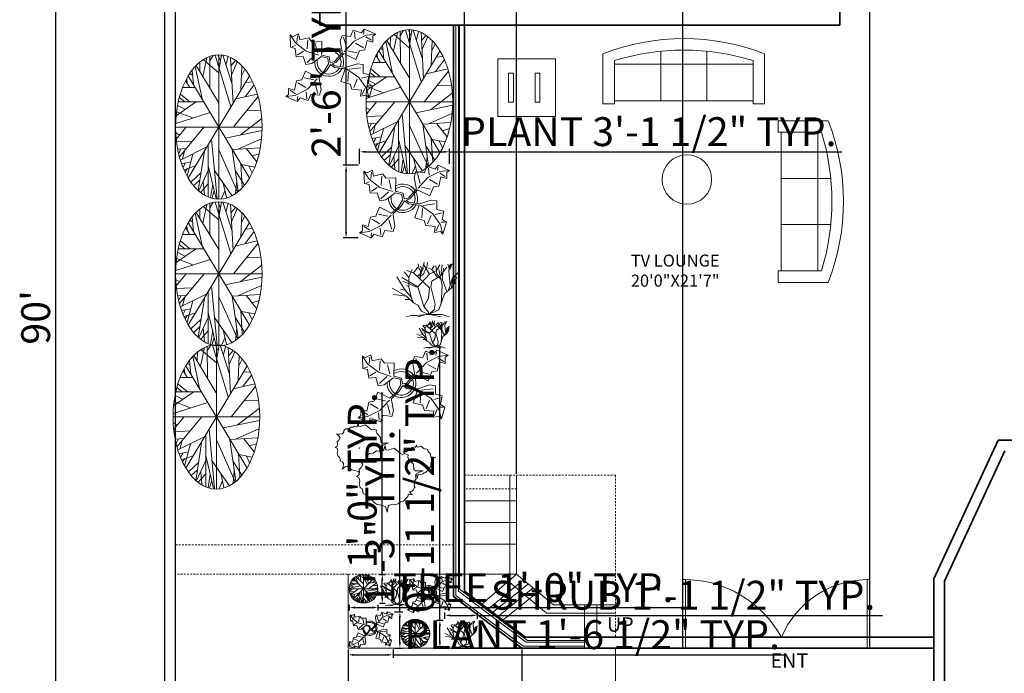
# Model space of a CAD drawing. Units: inches. Extents: x 2562 to 3392, y 1021 to 2243.
# Tile 2 of 6: x 2577 to 2986, y 1472 to 1744. Entities that reach past the tile are written whole.
import ezdxf

# ---------------------------------------------------------------- set-up
doc = ezdxf.new("R2010")
doc.units = ezdxf.units.IN
doc.linetypes.add('JIS_02_0.7', pattern=[1.35, 0.75, -0.6])
for name, color, linetype, lineweight in [('A-ANNO-DIMS', 2, 'Continuous', 18), ('A-ANNO-TEXT', 7, 'Continuous', 18), ('A-AREA-IDEN', 7, 'Continuous', 18), ('A-DOOR', 4, 'Continuous', 18), ('A-FLOR-STRS', 7, 'Continuous', 18), ('A-FLOR-STRS-HIDN', 8, 'JIS_02_0.7', 13), ('A-FURN', 8, 'Continuous', 18), ('A-GLAZ', 4, 'Continuous', 13), ('A-WALL', 7, 'Continuous', 35), ('C-PROP', 7, 'Continuous', 30), ('L-HRDS', 8, 'Continuous', 18), ('L-HRDS-HIDN', 8, 'JIS_02_0.7', 13), ('L-PLNT', 94, 'Continuous', 13)]:
    doc.layers.add(name, color=color, linetype=linetype, lineweight=lineweight)
doc.styles.get("Standard").update_dxf_attribs({"font": 'arial.ttf'})
doc.dimstyles.new('ISO-25', dxfattribs={"dimtxt": 12, "dimasz": 2.5, "dimexe": 1.25, "dimexo": 0.625, "dimtad": 1, "dimdec": 1, "dimlunit": 3, "dimtxsty": 'Standard', "dimcen": 2.5, "dimadec": 0, "dimazin": 0, "dimtfac": 1, "dimtdec": 1, "dimtmove": 0, "dimatfit": 3, "dimfxl": 1, "dimarcsym": 0})

# ---------------------------------------------------------------- blocks, each defined once
blk = doc.blocks.new('Sofa - Roundback 7 ft.')
for p, q in [((-12.00002, -32.4421), (-12.00003, -6.5971)), ((11.99997, -32.4421), (11.99998, -6.5971)), ((-36.000027, -34), (-36.000027, -11.4696)), ((-35.999844, -13.3819), (35.9998, -13.3819)), ((35.99998, -34), (35.99998, -11.4696)), ((-36.000027, -32.4421), (35.99998, -32.4421))]:
    blk.add_line(p, q)
for points in [[(-36.000027, -34), (-42.000027, -34), (-42.000027, -8)], [(41.99998, -8), (41.99998, -34), (35.99998, -34)]]:
    blk.add_lwpolyline(points)
for centre, radius, start, end in [((0, -114.25), 114.25, 68.43141, 111.5686), ((-0.00001, -127.1968), 121.1968, 72.72033, 107.2797)]:
    blk.add_arc(centre, radius, start, end)
blk = doc.blocks.new('Tree - deciduous plan')
for p, q in [((-22.0458, 42.0753), (-16.5881, 57.6486)), ((-12.5388, 54.9406), (-7.9613, 59.4546)), ((-12.3627, 32.1443), (-12.5388, 58.7776)), ((-5.3205, 59.6806), (16.5105, 16.7963)), ((2.426, 54.9406), (-1.4472, 59.9056)), ((0, 59.9996), (0, -60)), ((0.4894, 48.6208), (3.6584, 59.6806)), ((18.2711, 35.5298), (5.419, 59.6806)), ((9.8203, 51.5549), (12.8133, 58.5516)), ((19.6795, 19.5047), (16.3344, 57.6486)), ((-32.6092, 50.4264), (-23.2782, 23.5674)), ((-31.2008, 51.1035), (-0.2149, 20.1818)), ((-26.4472, 46.5894), (-26.2712, 53.8116)), ((-21.1656, 55.8436), (-0.0388, 45.0094)), ((17.0387, 51.1035), (23.2006, 55.1666)), ((17.7429, 43.6552), (25.4894, 54.2636)), ((31.6513, 50.8778), (30.2429, 30.5643)), ((42, 42), (-42, -42)), ((42, -42), (-42, 42)), ((-40.1797, 44.558), (-36.4825, 43.2038)), ((-37.0107, 47.0408), (-35.25, 35.5298)), ((31.1232, 42.5267), (35.8767, 48.1693)), ((-49.8627, 32.8214), (-32.7853, 32.8214)), ((-45.8134, 38.2383), (-40.5318, 33.0471)), ((-43.8768, 36.4326), (-44.405, 40.2696)), ((36.2288, 25.1474), (48.9049, 35.0784)), ((37.1091, 37.1098), (46.6161, 37.5612)), ((-53.2078, 27.4044), (-40.1797, 20.859)), ((54.3626, 25.3731), (20.9119, 0.3198)), ((23.3767, 23.3417), (53.3063, 27.4044)), ((-32.2571, 20.6333), (-59.1937, 9.348)), ((-57.081, 17.9248), (-47.0458, 14.7649)), ((-56.0247, 20.859), (-20.8134, 20.859)), ((-54.7923, 24.4702), (-47.75, 21.0847)), ((-59.7219, 2.8025), (-12.0106, 12.0565)), ((-58.6656, 12.7336), (-35.9543, 7.5424)), ((38.5175, 13.4107), (58.2359, 13.6364)), ((-54.6162, -24.7335), (-20.2853, 0.0941)), ((29.3626, -6.6771), (59.4682, 7.091)), ((-60, 0), (60, 0)), ((-59.7219, -4.8714), (-54.2641, -6.6771)), ((-45.2853, -0.1316), (-59.0177, -10.0627)), ((9.2922, -9.1598), (59.6443, -2.8401)), ((-58.4895, -12.3197), (-36.4825, -11.6426)), ((-14.8275, -15.0282), (-14.6515, -57.6865)), ((-10.074, -10.0627), (-2.5036, -59.7178)), ((26.3697, -18.4138), (58.9401, -9.8369)), ((-57.081, -18.4138), (-45.2853, -17.9624)), ((-52.6797, -18.188), (-55.4966, -22.0251)), ((-53.2078, -27.442), (-16.7641, -16.6081)), ((-47.2219, -19.3166), (-50.2148, -26.3135)), ((-35.9543, -22.4765), (-44.0529, -40.5329)), ((-19.9331, -20.2194), (-28.5599, -52.721)), ((-0.0388, -19.0909), (25.8415, -53.8495)), ((18.6232, -18.6394), (26.7218, -53.3981)), ((18.7992, -18.6394), (57.3556, -17.2853)), ((38.1654, -18.188), (52.426, -29.0219)), ((45.9119, -24.0564), (55.595, -22.2508)), ((-38.9472, -29.0219), (-51.4472, -30.6018)), ((-46.5177, -30.1504), (-49.5106, -33.536)), ((-32.4331, -32.4075), (-48.1021, -35.5674)), ((-14.6515, -32.1818), (-3.912, -59.4922)), ((30.419, -30.1504), (32.3556, -50.0125)), ((31.4753, -31.279), (49.6091, -33.3103)), ((41.5105, -32.6332), (46.088, -38.0501)), ((-43.7008, -34.6645), (-46.6937, -37.373)), ((-24.6867, -37.8244), (-38.7712, -45.7241)), ((-14.6515, -36.2445), (-27.6797, -52.9467)), ((-6.2008, -36.2445), (17.919, -57.0094)), ((22.8485, -36.4702), (35.3485, -48.4326)), ((-26.2712, -43.9185), (-34.7219, -48.6583)), ((-14.6515, -47.3041), (-25.0388, -54.3009)), ((-21.5177, -45.4984), (-19.9331, -56.1065)), ((-8.4895, -47.5298), (-11.4825, -58.5893)), ((5.9471, -46.6269), (10.5246, -58.5893)), ((24.7852, -44.8213), (23.0246, -54.978)), ((-6.3768, -52.721), (-9.3698, -58.815)), ((8.4119, -53.1724), (3.8344, -59.4922))]:
    blk.add_line(p, q)
blk.add_circle((0, 0), 60)
blk = doc.blocks.new('Plant - Rubber or Philodendron')
for p, q in [((8.8871, 10.7908), (9.9809, 13.4933)), ((9.9809, 13.4933), (13.3837, 12.301)), ((10.5828, 12.6946), (10.8893, 9.7953)), ((13.3837, 12.301), (14.68, 13.9039)), ((14.5816, 13.2037), (14.3848, 11.8033)), ((14.68, 13.9039), (19.3848, 11.8146)), ((-16.2005, 11.4774), (-13.9899, 8.1064)), ((-16.2005, 11.4774), (-14.8639, 10.7964)), ((-16.0159, 6.3329), (-16.2005, 11.4774)), ((-14.8639, 10.7964), (-12.6195, 11.8975)), ((-13.3174, 8.325), (-13.0735, 11.0065)), ((-12.6195, 11.8975), (-12.1909, 9.4345)), ((-12.1909, 9.4345), (-8.3829, 10.3)), ((-8.8369, 9.409), (-9.0894, 5.6095)), ((-8.3829, 10.3), (-7.0549, 8.501)), ((-7.0549, 8.501), (-3.0284, 8.6941)), ((-3.0284, 8.6941), (-3.0709, 3.1041)), ((4.6914, 8.8812), (5.3859, 11.2828)), ((4.6914, 8.8812), (5.5014, 4.4831)), ((5.3859, 11.2828), (8.8871, 10.7908)), ((5.9878, 10.4842), (7.1971, 6.3869)), ((10.3916, 8.7942), (6.2847, 4.4028)), ((15.3859, 11.3055), (10.3916, 8.7942)), ((15.7909, 9.1065), (14.8995, 5.3044)), ((15.2875, 10.6053), (17.5907, 9.2105)), ((19.3848, 11.8146), (15.3859, 11.3055)), ((18.1925, 8.4119), (15.7909, 9.1065)), ((19.3848, 11.8146), (18.1868, 10.9119)), ((18.1868, 10.9119), (18.1925, 8.4119)), ((-14.0069, 5.8704), (-16.0159, 6.3329)), ((-15.3434, 6.5514), (-13.9984, 6.9884)), ((-13.5868, 2.2894), (-14.0069, 5.8704)), ((-13.9899, 8.1064), (-9.5434, 4.7185)), ((-13.1329, 3.1804), (-10.6614, 4.727)), ((-9.5434, 4.7185), (-4.1917, 2.9888)), ((-4.8529, 4.012), (-5.7184, 7.82)), ((5.4346, 3.9146), (5.5014, 4.4831)), ((7.7005, 4.8881), (11.5025, 3.9967)), ((14.2977, 6.1031), (10.9934, 7.9956)), ((12.7005, 4.8994), (11.1089, 1.1958)), ((14.8995, 5.3044), (12.7005, 4.8994)), ((-10.6784, 2.491), (-13.5868, 2.2894)), ((-9.5858, -0.8715), (-10.6784, 2.491)), ((-9.1318, 0.0195), (-5.9793, 2.9025)), ((-7.1228, -0.443), (-3.5248, 2.2131)), ((-3.5248, 2.2131), (-3.3011, 2.4355)), ((-3.3011, 2.4355), (-0.5306, 1.7947)), ((-3.0709, 3.1041), (0.0797, 2.3163)), ((-0.5306, 1.7947), (-0.2255, -0.5527)), ((-0.5306, 1.7947), (-0.5306, 1.7947)), ((0.0797, 2.3163), (0.4866, -0.031)), ((0.4866, -0.031), (2.1141, 0.2298)), ((2.1141, 0.2298), (5.4346, 3.9146)), ((6.1032, 3.6844), (2.8262, -0.031)), ((11.1089, 1.1958), (6.1032, 3.6844)), ((-11.3237, -7.2629), (-9.7321, -3.5593)), ((-9.7321, -3.5593), (-4.7264, -6.0479)), ((-7.1228, -0.443), (-9.5858, -0.8715)), ((-2.019, -3.6148), (-4.7264, -6.0479)), ((-4.0579, -6.2781), (-0.9375, -3.1608)), ((-2.019, -3.6148), (-0.2255, -0.5527)), ((-0.9375, -3.1608), (0.5883, -0.8135)), ((0.5883, -0.8135), (2.2447, -2.0916)), ((2.8262, -0.031), (1.3003, -0.5527)), ((1.3003, -0.5527), (2.4193, -1.4655)), ((2.2447, -2.0916), (6.7108, -2.6626)), ((2.4193, -1.4655), (6.895, -2.1175)), ((4.943, -7.9659), (6.7108, -2.6626)), ((11.6605, -0.5413), (6.895, -2.1175)), ((12.3677, -6.1981), (7.219, -2.6772)), ((8.125, -4.0768), (7.7715, -7.9659)), ((8.3544, -2.7453), (13.1973, -2.1704)), ((11.6605, -0.5413), (14.1354, -0.8948)), ((14.1354, -0.8948), (14.1354, -4.4304)), ((-14.4141, -11.4699), (-13.5228, -7.6679)), ((-13.5228, -7.6679), (-11.3237, -7.2629)), ((-6.3237, -7.2516), (-10.1257, -6.3602)), ((-9.0148, -11.1577), (-4.9047, -6.8122)), ((-4.1246, -6.8466), (-4.0579, -6.2781)), ((-3.3146, -11.2447), (-4.1246, -6.8466)), ((8.8321, -9.0266), (4.943, -7.9659)), ((10.2463, -10.4408), (11.6605, -6.9053)), ((15.5496, -10.7943), (12.3677, -6.1981)), ((16.2567, -5.8446), (13.4283, -6.5517)), ((14.1354, -4.4304), (16.9638, -5.1375)), ((16.9638, -5.1375), (16.2567, -8.673)), ((-16.8157, -10.7754), (-14.4141, -11.4699)), ((-16.8101, -13.2754), (-16.8157, -10.7754)), ((-13.9107, -12.9688), (-16.2139, -11.574)), ((-14.0091, -13.669), (-9.0148, -11.1577)), ((-12.921, -8.4665), (-9.6166, -10.359)), ((-9.206, -15.0581), (-9.5126, -12.1588)), ((-4.611, -12.8477), (-5.8203, -8.7504)), ((-3.3146, -11.2447), (-4.0092, -13.6463)), ((9.5392, -11.1479), (8.8321, -9.0266)), ((13.4283, -11.5015), (9.5392, -11.1479)), ((13.0748, -13.9763), (13.4283, -11.5015)), ((14.8425, -10.7943), (13.7819, -13.2692)), ((16.6103, -14.6834), (15.5496, -10.7943)), ((17.3174, -9.7337), (15.9032, -9.7337)), ((16.2567, -8.673), (18.0245, -9.7337)), ((18.0245, -9.7337), (16.6103, -14.6834)), ((-18.008, -14.1781), (-16.8101, -13.2754)), ((-18.008, -14.1781), (-14.0091, -13.669)), ((-13.3032, -16.2674), (-18.008, -14.1781)), ((-12.0069, -14.6645), (-13.3032, -16.2674)), ((-13.2048, -15.5672), (-13.008, -14.1668)), ((-8.6042, -15.8568), (-12.0069, -14.6645)), ((-7.5103, -13.1543), (-8.6042, -15.8568)), ((-4.0092, -13.6463), (-7.5103, -13.1543)), ((15.5496, -13.6228), (13.0748, -13.9763)), ((16.6103, -14.6834), (15.5496, -13.6228))]:
    blk.add_line(p, q)
for centre, radius, start, end in [((0, 0), 6.1275, 34.37569, 120.1028), ((-0.0601, -0.2075), 5.2461, 33.82192, 124.9414), ((0.0308, 0.1664), 6, 178.6147, 235.1169), ((0.0308, 0.1664), 5, 168.1647, 238.6725), ((-0.2664, 0.1682), 5.2775, 338.4094, 20.03007), ((-0.098, 0.1364), 6.1288, 341.2017, 26.09184), ((-0.0234, 0.3825), 6.1492, 242.5812, 331.2714), ((-0.1102, 0.4886), 5.2883, 247.3711, 327.472)]:
    blk.add_arc(centre, radius, start, end)
blk = doc.blocks.new('Clump of Trees or Bushes - plan')
for points in [[(-10.993, 56.487), (-9.228, 58.426), (-10.144, 63.512), (-8.923, 67.033), (-3.43, 69.772), (2.673, 72.119), (-2.82, 71.728), (-10.449, 71.728), (-13.195, 74.075), (-13.806, 83.073), (-16.857, 86.594), (-22.045, 92.071), (-22.961, 94.81), (-22.656, 98.722), (-28.759, 100.678), (-31.811, 99.113), (-35.472, 101.461), (-45.543, 109.676), (-49.815, 108.503), (-55.308, 106.155), (-59.58, 106.938), (-60.801, 113.98), (-63.242, 104.982), (-67.209, 106.938), (-70.872, 104.59), (-74.839, 104.982), (-80.637, 101.461), (-86.435, 101.069), (-90.402, 97.548), (-90.402, 94.419), (-93.454, 90.898), (-98.947, 90.115), (-105.66, 90.115), (-101.083, 87.768), (-98.031, 82.682), (-100.778, 77.596), (-103.829, 74.466), (-103.219, 69.772), (-104.134, 65.077), (-108.102, 62.73), (-104.439, 60.774), (-102.609, 55.297), (-103.829, 50.211), (-102.303, 44.342), (-98.947, 41.995), (-98.031, 38.865), (-98.031, 34.953), (-93.148, 32.606), (-90.707, 29.476), (-91.317, 22.434), (-93.454, 17.348), (-89.487, 21.26), (-85.519, 23.999), (-82.468, 23.216), (-78.806, 19.304), (-74.228, 15.783), (-69.956, 15.392), (-59.886, 12.653), (-58.254, 7.074)], [(59.448, 5.262), (60.936, 4.858), (62.652, -1.011), (63.415, 4.858), (64.178, 5.836), (66.848, 6.814), (69.709, 6.569), (73.905, 7.792), (76.385, 9.748), (79.627, 10.237), (81.153, 12.438), (84.014, 15.127), (84.205, 17.084), (85.158, 17.573), (88.591, 16.839), (85.73, 20.262), (88.591, 20.751), (89.545, 21.974), (90.689, 24.174), (91.452, 24.663), (90.499, 25.886), (91.261, 31.999), (92.596, 33.466), (92.024, 36.645), (92.787, 38.845), (96.22, 40.557), (100.035, 42.024), (96.602, 41.779), (91.834, 41.779), (90.117, 43.246), (89.736, 48.871), (87.828, 51.071), (84.586, 54.494), (84.014, 56.206), (84.205, 58.651), (80.39, 59.873), (78.483, 58.895), (76.194, 60.362), (69.9, 65.497), (67.23, 64.764), (63.797, 63.297), (61.126, 63.786), (60.364, 68.187), (58.838, 62.563), (56.358, 63.786), (54.07, 62.319), (51.59, 62.563), (47.966, 60.362), (44.343, 60.118), (41.863, 57.917), (41.863, 55.961), (39.956, 53.761), (36.523, 53.272), (32.327, 53.272), (35.187, 51.805), (36.641, 49.381)]]:
    blk.add_lwpolyline(points)
for points in [[(-4.577, 66.508), (-7.629, 55.261), (-12.588, 57.706), (-17.166, 54.772), (-22.125, 55.261), (-29.372, 50.86), (-36.62, 50.371), (-41.579, 45.969), (-41.579, 42.057), (-45.393, 37.656), (-52.259, 36.678), (-60.651, 36.678), (-54.93, 33.743), (-51.115, 27.386), (-54.548, 21.029), (-58.363, 17.116), (-57.6, 11.248), (-58.744, 5.38), (-63.703, 2.446), (-59.126, 0), (-56.837, -6.846), (-58.363, -13.203), (-56.455, -20.539), (-52.259, -23.473), (-51.115, -27.385), (-51.115, -32.275), (-45.012, -35.21), (-41.96, -39.122), (-42.723, -47.924), (-45.393, -54.282), (-40.434, -49.391), (-35.475, -45.968), (-31.661, -46.946), (-27.083, -51.837), (-21.362, -56.238), (-16.021, -56.727), (-3.433, -60.15), (0, -71.887), (1.526, -60.15), (3.052, -58.194), (8.392, -56.238), (14.114, -56.727), (22.506, -54.282), (27.465, -50.369), (33.949, -49.391), (37.001, -44.99), (42.723, -39.611), (43.104, -35.699), (45.012, -34.721), (51.878, -36.188), (46.156, -29.341), (51.878, -28.363), (53.785, -25.918), (56.074, -21.517), (57.6, -20.539), (55.692, -18.094), (57.218, -5.868), (59.888, -2.934), (58.744, 3.424), (60.27, 7.825), (67.136, 11.248), (74.765, 14.182), (67.899, 13.693), (58.363, 13.693), (54.93, 16.627), (54.167, 27.875), (50.352, 32.276), (43.867, 39.123), (42.723, 42.546), (43.104, 47.436), (35.475, 49.882), (31.661, 47.925), (27.083, 50.86), (14.495, 61.129), (9.155, 59.662), (2.289, 56.728), (-3.052, 57.706)], [(-58.055, 61.947), (-58.97, 60.774), (-57.139, 60.774)], [(62.08, 35.667), (61.508, 34.933), (62.652, 34.933)], [(-1.144, 1.468), (-2.289, 0), (0, 0)]]:
    blk.add_lwpolyline(points, close=True)
blk = doc.blocks.new('Shrub - elevation')
for p, q in [((-14.88, 18.24), (-12.96, 20.64)), ((-12.471, 19.775), (-12.898, 22.044)), ((-11.28, 19.619), (-12.104, 21.184)), ((-11.433, 18.289), (-10.457, 22.749)), ((-8.16, 17.76), (-10.56, 21.6)), ((-9.48, 19.775), (-8.992, 22.592)), ((-7.2, 19.68), (-6.24, 21.12)), ((-5.086, 17.741), (-5.513, 21.34)), ((-5.28, 19.2), (-3.84, 21.6)), ((-3.84, 16.8), (-0.96, 20.64)), ((-3.377, 18.602), (-2.888, 21.575)), ((-0.508, 21.888), (-0.081, 20.558)), ((-0.203, 19.149), (0.102, 21.34)), ((-0.02, 20.01), (0.896, 21.105)), ((0.041, 20.714), (1.384, 22.044)), ((0.102, 21.34), (0.835, 21.888)), ((-18.24, 11.04), (-21.755, 16.655)), ((-16.8, 16.32), (-18.72, 18.72)), ((-14.88, 18.24), (-17.76, 19.2)), ((-16.8, 16.32), (-15.36, 19.68)), ((-8.16, 12), (-14.88, 18.24)), ((-13.325, 16.724), (-11.433, 18.289)), ((-12.96, 12.48), (-8.16, 17.76)), ((-11.677, 19.071), (-12.471, 19.775)), ((-12.043, 15.628), (-11.921, 18.836)), ((-11.982, 16.802), (-10.579, 18.054)), ((-11.921, 18.836), (-10.64, 20.401)), ((-10.579, 18.054), (-9.846, 19.697)), ((-7.2, 19.68), (-8.64, 20.16)), ((-8.16, 17.76), (-5.28, 19.2)), ((-4.8, 16.32), (-7.2, 19.68)), ((-7.2, 14.88), (-3.84, 16.8)), ((-3.377, 15.315), (-5.086, 17.819)), ((-2.88, 12.96), (-4.32, 19.68)), ((-2.766, 16.802), (-3.377, 18.602)), ((-2.88, 15.84), (-2.4, 20.16)), ((0.346, 13.203), (-0.203, 19.149)), ((-0.142, 19.384), (0.59, 20.401)), ((1.323, 16.254), (3.642, 18.289)), ((1.44, 15.36), (2.88, 17.28)), ((-12.96, 12.48), (-19.68, 16.32)), ((-13.92, 12.48), (-19.2, 14.88)), ((-16.8, 12.48), (-17.76, 12.96)), ((-16.8, 12.48), (-16.8, 16.32)), ((-15.84, 8.16), (-16.8, 12.48)), ((-12.96, 12.48), (-13.92, 12.48)), ((-10.56, 4.32), (-12.96, 12.48)), ((-7.68, 12.48), (-7.2, 14.88)), ((-6.72, 8.64), (-7.68, 12.48)), ((-3.36, 5.28), (-2.88, 12.96)), ((-0.96, 10.56), (-2.88, 15.84)), ((-0.48, 10.8), (0.346, 13.203)), ((0.346, 13.203), (1.323, 16.254)), ((0.96, 12), (1.44, 15.36)), ((0.96, 12), (2.88, 14.88)), ((1.92, 13.44), (2.4, 15.36)), ((2.4, 15.36), (3.36, 16.32)), ((-17.76, 8.64), (-23.663, 11.961)), ((-17.76, 8.64), (-23.128, 9.222)), ((-18.24, 11.04), (-20.16, 11.52)), ((-15.84, 8.16), (-18.24, 11.04)), ((-14.88, 5.76), (-17.76, 8.64)), ((-8.64, 7.68), (-8.16, 12)), ((-5.76, 5.28), (-6.72, 8.64)), ((-4.32, 2.88), (-1.92, 9.6)), ((-1.92, 9.6), (0.96, 12)), ((-16.32, 7.2), (-18.24, 7.2)), ((-14.88, 5.76), (-15.84, 8.16)), ((-12.96, 4.8), (-14.88, 5.76)), ((-11.52, 2.4), (-12.96, 4.8)), ((-10.56, 4.32), (-8.64, 7.68)), ((-8.64, 1.92), (-10.56, 4.32)), ((-6.24, 2.88), (-5.76, 5.28)), ((-15.84, 0.48), (-17.76, 0)), ((-13.44, 0.48), (-15.84, 0.48)), ((-9.6, 0.96), (-13.44, 0.48)), ((-9.6, 0.96), (-12.96, 0)), ((-8.64, 0.96), (-11.52, 2.4)), ((-9.6, 0.96), (-7.68, 0.96)), ((-8.64, 0.96), (-4.32, 2.88)), ((-8.64, 0.96), (-6.24, 2.88)), ((-8.64, 0.96), (-8.64, 1.92)), ((-8.64, 0.96), (-2.88, 0.96)), ((-7.68, 0.96), (-6.24, 0.48)), ((-6.24, 0.48), (-3.36, 0)), ((-2.88, 0.96), (0, 0))]:
    blk.add_line(p, q)
blk = doc.blocks.new('*D22')
at = {"layer": 'A-ANNO-DIMS', "color": 0, "lineweight": -2, "transparency": 16777216}
for p, q in [((2636.14, 2160.13), (2590.2, 2160.13)), ((2591.45, 2157.63), (2591.45, 1082.63)), ((2636.14, 1080.13), (2590.2, 1080.13))]:
    blk.add_line(p, q, dxfattribs=at)
at = {"layer": 'A-ANNO-DIMS', "color": 0, "transparency": 16777216}
for points in [[(2591.03, 2157.63), (2591.86, 2157.63), (2591.45, 2160.13)], [(2591.03, 1082.63), (2591.86, 1082.63), (2591.45, 1080.13)]]:
    blk.add_solid(points, dxfattribs=at)
at = {"layer": 'Defpoints', "color": 0, "transparency": 16777216}
for p in [(2636.76, 2160.13), (2591.45, 1080.13), (2636.76, 1080.13)]:
    blk.add_point(p, dxfattribs=at)
at = {"layer": 'A-ANNO-DIMS', "color": 0, "transparency": 16777216, "insert": (2584.7, 1620.13), "char_height": 12, "attachment_point": 5, "rotation": 90}
blk.add_mtext("90'", dxfattribs=at)
blk = doc.blocks.new('TABLE-END-24IN')
for p, q in [((0, 24), (24, 24)), ((0, 0), (0, 24)), ((24, 24), (24, 0)), ((4.5, 17.99), (6.5, 17.99)), ((4.5, 5.99), (4.5, 17.99)), ((6.5, 17.99), (6.5, 5.99)), ((15.56, 17.99), (17.56, 17.99)), ((15.56, 5.99), (15.56, 17.99)), ((17.56, 17.99), (17.56, 5.99)), ((6.5, 5.99), (4.5, 5.99)), ((17.56, 5.99), (15.56, 5.99)), ((24, 0), (0, 0))]:
    blk.add_line(p, q)
blk = doc.blocks.new('*D55')
at = {"layer": 'A-ANNO-DIMS', "color": 0, "lineweight": -2, "transparency": 16777216}
for p, q in [((2713.35, 1500.64), (2713.35, 1498.22)), ((2715.85, 1499.47), (2722.85, 1499.47)), ((2725.35, 1500.64), (2725.35, 1498.22)), ((2725.35, 1499.47), (2851.91, 1499.47))]:
    blk.add_line(p, q, dxfattribs=at)
at = {"layer": 'A-ANNO-DIMS', "color": 0, "transparency": 16777216}
for points in [[(2715.85, 1499.89), (2715.85, 1499.05), (2713.35, 1499.47)], [(2722.85, 1499.89), (2722.85, 1499.05), (2725.35, 1499.47)]]:
    blk.add_solid(points, dxfattribs=at)
at = {"layer": 'Defpoints', "color": 0, "transparency": 16777216}
for p in [(2713.35, 1501.27), (2725.35, 1501.27), (2725.35, 1499.47)]:
    blk.add_point(p, dxfattribs=at)
at = {"layer": 'A-ANNO-DIMS', "color": 0, "transparency": 16777216, "insert": (2789.88, 1506.22), "char_height": 12, "attachment_point": 5}
blk.add_mtext('TREE 1\'-0" TYP.', dxfattribs=at)
blk = doc.blocks.new('*D56')
at = {"layer": 'A-ANNO-DIMS', "color": 0, "lineweight": -2, "transparency": 16777216}
for p, q in [((2727.15, 1513.27), (2727.15, 1589.04)), ((2725.97, 1513.27), (2728.4, 1513.27)), ((2727.15, 1503.77), (2727.15, 1510.77)), ((2725.97, 1501.27), (2728.4, 1501.27))]:
    blk.add_line(p, q, dxfattribs=at)
at = {"layer": 'A-ANNO-DIMS', "color": 0, "transparency": 16777216}
for points in [[(2726.73, 1510.77), (2727.56, 1510.77), (2727.15, 1513.27)], [(2726.73, 1503.77), (2727.56, 1503.77), (2727.15, 1501.27)]]:
    blk.add_solid(points, dxfattribs=at)
at = {"layer": 'Defpoints', "color": 0, "transparency": 16777216}
for p in [(2725.35, 1513.27), (2727.15, 1513.27), (2725.35, 1501.27)]:
    blk.add_point(p, dxfattribs=at)
at = {"layer": 'A-ANNO-DIMS', "color": 0, "transparency": 16777216, "insert": (2720.39, 1552.4), "char_height": 12, "attachment_point": 5, "rotation": 90}
blk.add_mtext('1\'-0" TYP.', dxfattribs=at)
blk = doc.blocks.new('*D59')
at = {"layer": 'A-ANNO-DIMS', "color": 0, "lineweight": -2, "transparency": 16777216}
for p, q in [((2753.12, 1494.79), (2753.12, 1497.46)), ((2766.77, 1494.79), (2766.77, 1497.46)), ((2755.62, 1496.21), (2764.27, 1496.21)), ((2766.77, 1496.21), (2934.91, 1496.21))]:
    blk.add_line(p, q, dxfattribs=at)
at = {"layer": 'A-ANNO-DIMS', "color": 0, "transparency": 16777216}
for points in [[(2755.62, 1496.63), (2755.62, 1495.8), (2753.12, 1496.21)], [(2764.27, 1496.63), (2764.27, 1495.8), (2766.77, 1496.21)]]:
    blk.add_solid(points, dxfattribs=at)
at = {"layer": 'Defpoints', "color": 0, "transparency": 16777216}
for p in [(2753.12, 1494.16), (2766.77, 1496.21), (2766.77, 1494.16)]:
    blk.add_point(p, dxfattribs=at)
at = {"layer": 'A-ANNO-DIMS', "color": 0, "transparency": 16777216, "insert": (2852.09, 1503.04), "char_height": 12, "attachment_point": 5}
blk.add_mtext('SHRUB 1\'-1 1/2" TYP.', dxfattribs=at)
blk = doc.blocks.new('*D60')
at = {"layer": 'A-ANNO-DIMS', "color": 0, "lineweight": -2, "transparency": 16777216}
for p, q in [((2751.07, 1494.16), (2751.07, 1608.35)), ((2752.5, 1494.16), (2749.82, 1494.16)), ((2751.07, 1485.29), (2751.07, 1491.66)), ((2752.5, 1482.79), (2749.82, 1482.79))]:
    blk.add_line(p, q, dxfattribs=at)
at = {"layer": 'A-ANNO-DIMS', "color": 0, "transparency": 16777216}
for points in [[(2750.66, 1491.66), (2751.49, 1491.66), (2751.07, 1494.16)], [(2750.66, 1485.29), (2751.49, 1485.29), (2751.07, 1482.79)]]:
    blk.add_solid(points, dxfattribs=at)
at = {"layer": 'Defpoints', "color": 0, "transparency": 16777216}
for p in [(2751.07, 1494.16), (2753.12, 1494.16), (2753.12, 1482.79)]:
    blk.add_point(p, dxfattribs=at)
at = {"layer": 'A-ANNO-DIMS', "color": 0, "transparency": 16777216, "insert": (2744.24, 1552.51), "char_height": 12, "attachment_point": 5, "rotation": 90}
blk.add_mtext('0\'-11 1/2" TYP.', dxfattribs=at)
blk = doc.blocks.new('*D65')
at = {"layer": 'A-ANNO-DIMS', "color": 0, "lineweight": -2, "transparency": 16777216}
for p, q in [((2717.73, 1683.95), (2717.73, 1690.19)), ((2755.13, 1683.95), (2755.13, 1690.19)), ((2720.23, 1688.94), (2752.63, 1688.94)), ((2755.13, 1688.94), (2918.08, 1688.94))]:
    blk.add_line(p, q, dxfattribs=at)
at = {"layer": 'A-ANNO-DIMS', "color": 0, "transparency": 16777216}
for points in [[(2720.23, 1689.35), (2720.23, 1688.52), (2717.73, 1688.94)], [(2752.63, 1689.35), (2752.63, 1688.52), (2755.13, 1688.94)]]:
    blk.add_solid(points, dxfattribs=at)
at = {"layer": 'Defpoints', "color": 0, "transparency": 16777216}
for p in [(2755.13, 1688.94), (2717.73, 1683.33), (2755.13, 1683.33)]:
    blk.add_point(p, dxfattribs=at)
at = {"layer": 'A-ANNO-DIMS', "color": 0, "transparency": 16777216, "insert": (2837.85, 1695.77), "char_height": 12, "attachment_point": 5}
blk.add_mtext('PLANT 3\'-1 1/2" TYP.', dxfattribs=at)
blk = doc.blocks.new('*D66')
at = {"layer": 'A-ANNO-DIMS', "color": 0, "lineweight": -2, "transparency": 16777216}
for p, q in [((2712.12, 1683.33), (2712.12, 1760.43)), ((2717.11, 1683.33), (2710.87, 1683.33)), ((2712.12, 1655.66), (2712.12, 1680.83)), ((2717.11, 1653.16), (2710.87, 1653.16))]:
    blk.add_line(p, q, dxfattribs=at)
at = {"layer": 'A-ANNO-DIMS', "color": 0, "transparency": 16777216}
for points in [[(2711.71, 1680.83), (2712.54, 1680.83), (2712.12, 1683.33)], [(2711.71, 1655.66), (2712.54, 1655.66), (2712.12, 1653.16)]]:
    blk.add_solid(points, dxfattribs=at)
at = {"layer": 'Defpoints', "color": 0, "transparency": 16777216}
for p in [(2712.12, 1683.33), (2717.73, 1683.33), (2717.73, 1653.16)]:
    blk.add_point(p, dxfattribs=at)
at = {"layer": 'A-ANNO-DIMS', "color": 0, "transparency": 16777216, "insert": (2705.37, 1723.13), "char_height": 12, "attachment_point": 5, "rotation": 90}
blk.add_mtext('2\'-6" TYP.', dxfattribs=at)
blk = doc.blocks.new('*D67')
at = {"layer": 'A-ANNO-DIMS', "color": 0, "lineweight": -2, "transparency": 16777216}
for p, q in [((2712.95, 1482.01), (2712.95, 1478.58)), ((2731.65, 1482.01), (2731.65, 1478.58)), ((2715.45, 1479.83), (2729.15, 1479.83)), ((2731.65, 1479.83), (2894.6, 1479.83))]:
    blk.add_line(p, q, dxfattribs=at)
at = {"layer": 'A-ANNO-DIMS', "color": 0, "transparency": 16777216}
for points in [[(2715.45, 1480.24), (2715.45, 1479.41), (2712.95, 1479.83)], [(2729.15, 1480.24), (2729.15, 1479.41), (2731.65, 1479.83)]]:
    blk.add_solid(points, dxfattribs=at)
at = {"layer": 'Defpoints', "color": 0, "transparency": 16777216}
for p in [(2712.95, 1482.63), (2731.65, 1482.63), (2731.65, 1479.83)]:
    blk.add_point(p, dxfattribs=at)
at = {"layer": 'A-ANNO-DIMS', "color": 0, "transparency": 16777216, "insert": (2814.37, 1486.66), "char_height": 12, "attachment_point": 5}
blk.add_mtext('PLANT 1\'-6 1/2" TYP.', dxfattribs=at)
blk = doc.blocks.new('*D68')
at = {"layer": 'A-ANNO-DIMS', "color": 0, "lineweight": -2, "transparency": 16777216}
for p, q in [((2734.45, 1497.72), (2734.45, 1573.48)), ((2732.27, 1497.72), (2735.7, 1497.72)), ((2734.45, 1485.13), (2734.45, 1495.22)), ((2732.27, 1482.63), (2735.7, 1482.63))]:
    blk.add_line(p, q, dxfattribs=at)
at = {"layer": 'A-ANNO-DIMS', "color": 0, "transparency": 16777216}
for points in [[(2734.04, 1495.22), (2734.87, 1495.22), (2734.45, 1497.72)], [(2734.04, 1485.13), (2734.87, 1485.13), (2734.45, 1482.63)]]:
    blk.add_solid(points, dxfattribs=at)
at = {"layer": 'Defpoints', "color": 0, "transparency": 16777216}
for p in [(2731.65, 1497.72), (2734.45, 1497.72), (2731.65, 1482.63)]:
    blk.add_point(p, dxfattribs=at)
at = {"layer": 'A-ANNO-DIMS', "color": 0, "transparency": 16777216, "insert": (2727.7, 1536.85), "char_height": 12, "attachment_point": 5, "rotation": 90}
blk.add_mtext('1\'-3" TYP.', dxfattribs=at)
blk = doc.blocks.new('*D74')
at = {"layer": 'A-ANNO-DIMS', "color": 0, "lineweight": -2, "transparency": 16777216}
for p, q in [((2852.07, 1483.26), (2852.07, 2219.58)), ((2854.57, 2218.33), (2927.14, 2218.33)), ((2929.64, 1483.26), (2929.64, 2219.58))]:
    blk.add_line(p, q, dxfattribs=at)
at = {"layer": 'A-ANNO-DIMS', "color": 0, "transparency": 16777216}
for points in [[(2854.57, 2218.75), (2854.57, 2217.92), (2852.07, 2218.33)], [(2927.14, 2218.75), (2927.14, 2217.92), (2929.64, 2218.33)]]:
    blk.add_solid(points, dxfattribs=at)
at = {"layer": 'Defpoints', "color": 0, "transparency": 16777216}
for p in [(2929.64, 2218.33), (2852.07, 1482.63), (2929.64, 1482.63)]:
    blk.add_point(p, dxfattribs=at)
at = {"layer": 'A-ANNO-DIMS', "color": 0, "transparency": 16777216, "insert": (2890.85, 2225.16), "char_height": 12, "attachment_point": 5}
blk.add_mtext('6\'-5 1/2"', dxfattribs=at)
blk = doc.blocks.new('*D78')
at = {"layer": 'A-ANNO-DIMS', "color": 0, "lineweight": -2, "transparency": 16777216}
for p, q in [((2712.95, 1482.01), (2712.95, 1020.68)), ((2785.11, 1482.01), (2785.11, 1020.68)), ((2715.45, 1021.93), (2782.61, 1021.93))]:
    blk.add_line(p, q, dxfattribs=at)
at = {"layer": 'A-ANNO-DIMS', "color": 0, "transparency": 16777216}
for points in [[(2715.45, 1022.35), (2715.45, 1021.52), (2712.95, 1021.93)], [(2782.61, 1022.35), (2782.61, 1021.52), (2785.11, 1021.93)]]:
    blk.add_solid(points, dxfattribs=at)
at = {"layer": 'Defpoints', "color": 0, "transparency": 16777216}
for p in [(2712.95, 1482.63), (2785.11, 1482.63), (2785.11, 1021.93)]:
    blk.add_point(p, dxfattribs=at)
at = {"layer": 'A-ANNO-DIMS', "color": 0, "transparency": 16777216, "insert": (2749.03, 1028.68), "char_height": 12, "attachment_point": 5}
blk.add_mtext('6\'-0"', dxfattribs=at)
blk = doc.blocks.new('*D79')
at = {"layer": 'A-ANNO-DIMS', "color": 0, "lineweight": -2, "transparency": 16777216}
for p, q in [((2761.26, 1555.09), (2761.26, 2219.58)), ((2763.76, 2218.33), (2780.46, 2218.33)), ((2782.96, 1555.09), (2782.96, 2219.58)), ((2782.96, 2218.33), (2845.44, 2218.33))]:
    blk.add_line(p, q, dxfattribs=at)
at = {"layer": 'A-ANNO-DIMS', "color": 0, "transparency": 16777216}
for points in [[(2763.76, 2218.75), (2763.76, 2217.92), (2761.26, 2218.33)], [(2780.46, 2218.75), (2780.46, 2217.92), (2782.96, 2218.33)]]:
    blk.add_solid(points, dxfattribs=at)
at = {"layer": 'Defpoints', "color": 0, "transparency": 16777216}
for p in [(2782.96, 2218.33), (2761.26, 1554.47), (2782.96, 1554.47)]:
    blk.add_point(p, dxfattribs=at)
at = {"layer": 'A-ANNO-DIMS', "color": 0, "transparency": 16777216, "insert": (2815.45, 2225.16), "char_height": 12, "attachment_point": 5}
blk.add_mtext('1\'-9 1/2"', dxfattribs=at)

msp = doc.modelspace()

# ---------------------------------------------------------------- linework, layer by layer
at = {"layer": 'A-DOOR'}
for p, q in [((2853.07, 1511.13), (2852.07, 1511.13)), ((2852.07, 1511.13), (2852.07, 1482.63)), ((2853.07, 1487.13), (2853.07, 1511.13)), ((2929.64, 1511.13), (2928.64, 1511.13)), ((2928.64, 1511.13), (2928.64, 1482.63)), ((2929.64, 1487.13), (2929.64, 1511.13)), ((2853.07, 1482.63), (2853.07, 1487.13)), ((2929.64, 1482.63), (2929.64, 1487.13))]:
    msp.add_line(p, q, dxfattribs=at)
for centre, radius, start, end in [((2852.57, 1465.16), 45.97, 28.5464, 90.6232), ((2929.14, 1471.86), 39.27, 89.2706, 157.1178)]:
    msp.add_arc(centre, radius, start, end, dxfattribs=at)
at = {"layer": 'A-FLOR-STRS'}
for p, q in [((2780.08, 1509.94), (2780.08, 1554.47)), ((2782.96, 1513.4), (2782.96, 1554.47)), ((2761.26, 1543.85), (2782.96, 1543.85)), ((2761.26, 1534.85), (2782.96, 1534.85)), ((2761.26, 1525.85), (2782.96, 1525.85)), ((2736.95, 1513.4), (2782.96, 1513.4)), ((2782.96, 1513.4), (2768.48, 1500.84)), ((2785.85, 1511), (2771.09, 1498.86)), ((2795.43, 1497.2), (2780.08, 1509.94)), ((2798.3, 1500.66), (2782.96, 1513.4)), ((2787.85, 1509.34), (2773, 1497.42)), ((2789.87, 1507.67), (2775.27, 1495.7)), ((2791.9, 1505.98), (2777.21, 1494.24)), ((2795.43, 1497.2), (2824.1, 1497.2)), ((2824.1, 1500.66), (2798.3, 1500.66)), ((2798.3, 1500.66), (2798.3, 1500.66)), ((2811.2, 1500.66), (2811.2, 1487.13)), ((2816.22, 1500.66), (2816.22, 1487.13)), ((2811.2, 1487.13), (2811.2, 1482.63))]:
    msp.add_line(p, q, dxfattribs=at)
at = {"layer": 'A-FLOR-STRS-HIDN'}
for p, q in [((2824.1, 1554.47), (2761.26, 1554.47)), ((2824.1, 1554.47), (2824.1, 1487.13)), ((2782.96, 1548.9), (2761.26, 1548.9))]:
    msp.add_line(p, q, dxfattribs=at)
at = {"layer": 'A-FURN'}
msp.add_circle((2853.69, 1677.44), 10.29, dxfattribs=at)
at = {"layer": 'A-GLAZ'}
for p, q in [((2757.76, 1504.54), (2757.76, 1741.63)), ((2758.76, 1506.29), (2758.76, 1741.63)), ((2759.26, 1507.17), (2759.26, 1741.63)), ((2786.92, 1485.03), (2758.76, 1506.29)), ((2787.52, 1485.82), (2759.26, 1507.17)), ((2785.71, 1483.43), (2757.76, 1504.54)), ((2786.92, 1485.03), (2811.2, 1485.03)), ((2787.52, 1485.82), (2811.2, 1485.82)), ((2785.71, 1483.43), (2811.2, 1483.43))]:
    msp.add_line(p, q, dxfattribs=at)
at = {"layer": 'A-WALL'}
for p, q in [((2701.26, 1741.63), (2701.26, 2095.63)), ((2917.26, 1741.63), (2917.26, 1794.5)), ((2701.26, 1741.63), (2917.26, 1741.63)), ((2756.76, 1504.05), (2756.76, 1741.63)), ((2756.76, 1504.05), (2756.76, 1741.63)), ((2761.26, 1506.29), (2761.26, 1741.63)), ((2956.26, 1511.43), (2982.95, 1569.13)), ((2982.95, 1569.13), (3072.12, 1569.13)), ((2960.76, 1510.44), (2985.83, 1564.63)), ((2956.26, 1500.7), (2956.26, 1511.43)), ((2960.76, 1510.44), (2960.76, 1442.58)), ((2786.62, 1487.13), (2761.26, 1506.29)), ((2785.11, 1482.63), (2756.76, 1504.05)), ((2956.26, 1500.7), (2956.26, 1441.58)), ((2956.26, 1487.13), (2786.62, 1487.13)), ((2756.76, 1482.63), (2917.26, 1482.63)), ((2956.26, 1482.63), (2756.76, 1482.63)), ((2917.26, 1482.63), (2956.26, 1482.63))]:
    msp.add_line(p, q, dxfattribs=at)
at = {"layer": 'C-PROP'}
for p, q in [((2636.76, 1080.13), (2636.76, 2160.13)), ((2641.26, 1084.63), (2641.26, 2155.63))]:
    msp.add_line(p, q, dxfattribs=at)
at = {"layer": 'L-HRDS'}
for p, q in [((2712.95, 1482.63), (2712.95, 1513.4)), ((2756.76, 1482.63), (2712.95, 1482.63)), ((2824.1, 1482.63), (2824.1, 1375.08))]:
    msp.add_line(p, q, dxfattribs=at)
at = {"layer": 'L-HRDS-HIDN'}
for p, q in [((2756.76, 1525.51), (2641.26, 1525.51)), ((2710.26, 1513.4), (2641.26, 1513.4)), ((2736.95, 1513.4), (2710.26, 1513.4))]:
    msp.add_line(p, q, dxfattribs=at)

# ---------------------------------------------------------------- block references
at = {"layer": 'A-FURN', "xscale": 0.8, "yscale": 0.8}
msp.add_blockref('Sofa - Roundback 7 ft.', (2852.4, 1736.04), dxfattribs=at)
at = {"layer": 'A-FURN'}
msp.add_blockref('TABLE-END-24IN', (2775.11, 1703.6), dxfattribs=at)
at = {"layer": 'A-FURN', "xscale": 0.8, "yscale": 0.8, "rotation": 270}
msp.add_blockref('Sofa - Roundback 7 ft.', (2918.76, 1668.28), dxfattribs=at)
at = {"layer": 'L-PLNT'}
for name, p in [('Plant - Rubber or Philodendron', (2705.03, 1726.09)), ('Plant - Rubber or Philodendron', (2735.74, 1669.43)), ('Shrub - elevation', (2754.94, 1620.36, 1)), ('Plant - Rubber or Philodendron', (2735.08, 1592.58))]:
    msp.add_blockref(name, p, dxfattribs=at)
for name, p, xscale, yscale in [('Tree - deciduous plan', (2738.39, 1709.73, 1), 0.3, 0.5), ('Tree - deciduous plan', (2659.26, 1699.26, 1), 0.3, 0.5), ('Tree - deciduous plan', (2659.26, 1638.22, 1), 0.3, 0.5), ('Shrub - elevation', (2753.3, 1607.33, 1), 0.5, 0.5), ('Tree - deciduous plan', (2658.23, 1578.72, 1), 0.3, 0.5), ('Clump of Trees or Bushes - plan', (2729.23, 1553.52), 0.2, 0.2), ('Tree - deciduous plan', (2719.35, 1507.27, 1), 0.1, 0.1), ('Shrub - elevation', (2737.22, 1500.21, 1), 0.5, 0.5), ('Plant - Rubber or Philodendron', (2746.63, 1505.58), 0.5, 0.5), ('Plant - Rubber or Philodendron', (2721.96, 1490.77), 0.5, 0.5), ('Tree - deciduous plan', (2740.86, 1488.63, 1), 0.1, 0.1), ('Shrub - elevation', (2764.95, 1482.79, 1), 0.5, 0.5)]:
    msp.add_blockref(name, p, dxfattribs=dict(at, xscale=xscale, yscale=yscale))

# ---------------------------------------------------------------- texts
at = {"layer": 'A-ANNO-TEXT', "char_height": 6, "attachment_point": 1}
for s, insert in [('UP', (2820.49, 1495.42)), ('ENT', (2888.44, 1480.44))]:
    msp.add_mtext_dynamic_manual_height_columns(s, width=2.4229, gutter_width=12.5, heights=[0], dxfattribs=dict(at, insert=insert))
at = {"layer": 'A-AREA-IDEN', "insert": (2830.41, 1646.23), "char_height": 5, "attachment_point": 1}
msp.add_mtext('TV LOUNGE \\P20\'0"X21\'7"', dxfattribs=at)

# ---------------------------------------------------------------- dimensions: what is measured, and where the dimension line sits
at = {"layer": 'A-ANNO-DIMS'}
for base, p1, p2, picture, middle in [((2782.96, 2218.33), (2761.26, 1554.47), (2782.96, 1554.47), '*D79', (2815.45, 2225.16)), ((2929.64, 2218.33), (2852.07, 1482.63), (2929.64, 1482.63), '*D74', (2890.85, 2225.16)), ((2785.11, 1021.93), (2712.95, 1482.63), (2785.11, 1482.63), '*D78', (2749.03, 1028.68))]:
    dim = msp.add_linear_dim(base=base, p1=p1, p2=p2, dimstyle='ISO-25', override={"dimdec": 1, "dimlfac": 1, "dimrnd": 0, "dimzin": 1, "dimdsep": 46, "dimlunit": 4, "dimfrac": 2}, dxfattribs=at)
    dim.commit()
    dim.dimension.update_dxf_attribs({"geometry": picture, "text_midpoint": middle})
dim = msp.add_linear_dim(base=(2591.45, 1080.13), p1=(2636.76, 2160.13), p2=(2636.76, 1080.13), angle=90, dimstyle='ISO-25', override={"dimclrd": 0, "dimclre": 0, "dimclrt": 0}, dxfattribs=at)
dim.commit()
dim.dimension.update_dxf_attribs({"geometry": '*D22', "text_midpoint": (2584.7, 1620.13)})
for base, p1, p2, picture, middle in [((2712.12, 1683.33), (2717.73, 1653.16), (2717.73, 1683.33), '*D66', (2705.37, 1723.13)), ((2751.07, 1494.16), (2753.12, 1482.79), (2753.12, 1494.16), '*D60', (2744.24, 1552.51)), ((2727.15, 1513.27), (2725.35, 1501.27), (2725.35, 1513.27), '*D56', (2720.39, 1552.4)), ((2734.45, 1497.72), (2731.65, 1482.63), (2731.65, 1497.72), '*D68', (2727.7, 1536.85))]:
    dim = msp.add_linear_dim(base=base, p1=p1, p2=p2, angle=90, text='<> TYP.', dimstyle='ISO-25', override={"dimdec": 1, "dimlfac": 1, "dimrnd": 0, "dimzin": 1, "dimdsep": 46, "dimlunit": 4, "dimfrac": 2}, dxfattribs=at)
    dim.commit()
    dim.dimension.update_dxf_attribs({"geometry": picture, "text_midpoint": middle})
for base, p1, p2, text, picture, middle in [((2755.13, 1688.94), (2717.73, 1683.33), (2755.13, 1683.33), 'PLANT <> TYP.', '*D65', (2837.85, 1695.77)), ((2766.7738, 1496.2124), (2753.1213, 1494.1645), (2766.7738, 1494.1645), 'SHRUB <> TYP.', '*D59', (2852.0939, 1503.042)), ((2725.35, 1499.47), (2713.35, 1501.27), (2725.35, 1501.27), 'TREE <> TYP.', '*D55', (2789.88, 1506.22)), ((2731.65, 1479.83), (2712.95, 1482.63), (2731.65, 1482.63), 'PLANT <> TYP.', '*D67', (2814.37, 1486.66))]:
    dim = msp.add_linear_dim(base=base, p1=p1, p2=p2, text=text, dimstyle='ISO-25', override={"dimdec": 1, "dimlfac": 1, "dimrnd": 0, "dimzin": 1, "dimdsep": 46, "dimlunit": 4, "dimfrac": 2}, dxfattribs=at)
    dim.commit()
    dim.dimension.update_dxf_attribs({"geometry": picture, "text_midpoint": middle})

doc.saveas('drawing.dxf')
